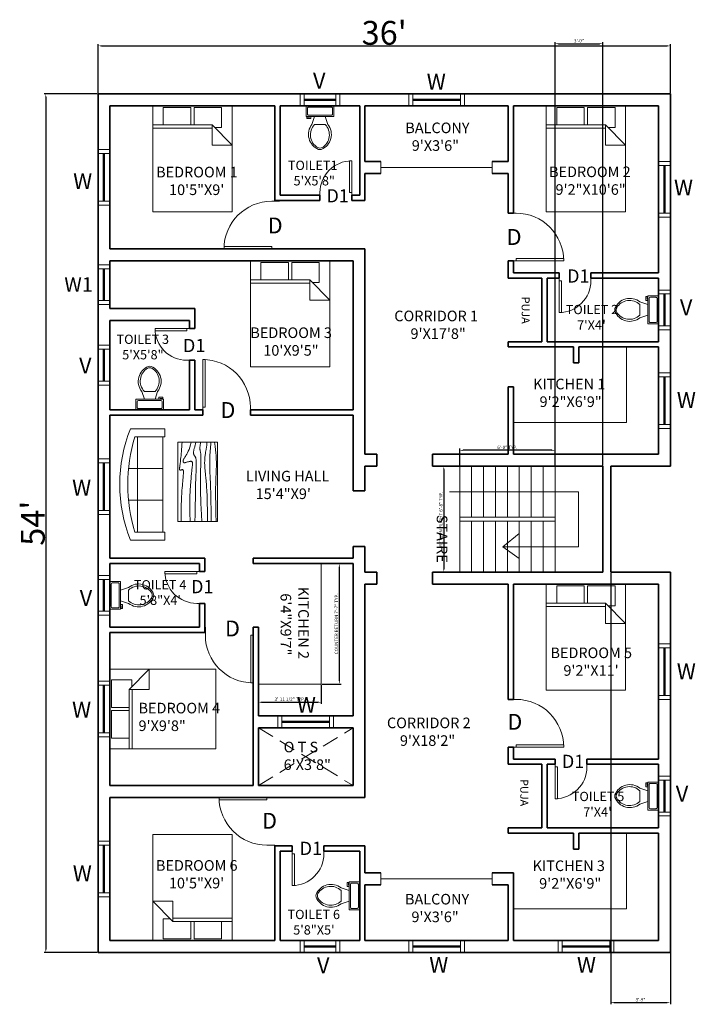
# Model space of a CAD drawing. Units: inches. Extents: x 2391 to 16591, y 7259 to 10239.
# Tile 26 of 27: x 14913 to 15423, y 9413 to 10156. Entities that reach past the tile are written whole.
import ezdxf

# ---------------------------------------------------------------- set-up
doc = ezdxf.new("R2010")
doc.units = ezdxf.units.IN
doc.linetypes.add('DASHED', pattern=[19.05, 12.7, -6.35])
for name, color, linetype, lineweight in [('A-ANNO-DIMS', 4, 'Continuous', 18), ('A-ANNO-IDEN', 2, 'Continuous', 18), ('A-ANNO-SYMB', 3, 'Continuous', 18), ('A-AREA-IDEN', 7, 'Continuous', 18), ('A-DOOR', 3, 'Continuous', 18), ('A-FLOR-CASE', 6, 'Continuous', 18), ('A-FLOR-FIXT', 9, 'Continuous', 18), ('A-FLOR-HRAL', 8, 'Continuous', 18), ('A-FLOR-OPEN', 4, 'DASHED', 13), ('A-FLOR-STRS', 7, 'Continuous', 18), ('A-FURN', 8, 'Continuous', 18), ('A-GLAZ', 4, 'Continuous', 18), ('A-WALL', 7, 'Continuous', 35)]:
    doc.layers.add(name, color=color, linetype=linetype, lineweight=lineweight)
doc.styles.get("Standard").update_dxf_attribs({"font": 'arial.ttf'})
doc.dimstyles.new('ISO-25', dxfattribs={"dimtxt": 2.5, "dimasz": 2.5, "dimexe": 1.25, "dimexo": 0.625, "dimtad": 1, "dimdec": 0, "dimlunit": 3, "dimtxsty": 'Standard', "dimcen": 2.5, "dimadec": 0, "dimazin": 0, "dimtfac": 1, "dimtdec": 0, "dimtmove": 0, "dimatfit": 3, "dimfxl": 1, "dimarcsym": 0})

# ---------------------------------------------------------------- blocks, each defined once
blk = doc.blocks.new('Bed - Queen')
for p, q in [((0, -80.00003), (0, 0)), ((0, 0), (59.99999, 0)), ((59.99999, 0), (59.99999, -80.00003)), ((7.99999, -1.2), (28.79998, -1.2)), ((7.99999, -14.4), (7.99999, -1.2)), ((28.79998, -1.2), (28.79998, -14.4)), ((31.19999, -1.2), (51.99999, -1.2)), ((31.19999, -14.4), (31.19999, -1.2)), ((51.99999, -1.2), (51.99999, -16.4)), ((0, -14.4), (44.8, -14.4)), ((59.99999, -29.6), (44.8, -14.4)), ((44.8, -14.4), (44.8, -29.6)), ((44.8, -16.8), (0, -16.8)), ((51.99999, -16.4), (46.79936, -16.4)), ((44.8, -29.6), (59.99999, -29.6)), ((59.99999, -80.00003), (0, -80.00003))]:
    blk.add_line(p, q)
blk = doc.blocks.new('Toilet - top')
for p, q in [((9.5, -6), (9.5, -2)), ((-10, -8.5), (-8, -8.5)), ((-10, -9.5), (-10, -8.5)), ((-7, -9.5), (-10, -9.5)), ((-8, -8.5), (-8, -8)), ((-7, -8), (-7, -9.5)), ((-4, -8), (-6, -14)), ((4, -14), (-4, -14)), ((4, -8), (6, -14))]:
    blk.add_line(p, q)
blk.add_lwpolyline([(10.5, -8), (10.5, 0), (-10.5, 0), (-10.5, -8)], close=True)
for points in [[(-9.5, -2), (-9.5, -6)], [(8.5, -1), (-8.5, -1)], [(-8.5, -7), (8.5, -7)]]:
    blk.add_lwpolyline(points)
for centre, radius, start, end in [((-8.62, -1.88), 0.884, 81.8699, 188.1301), ((-8.62, -6.12), 0.884, 171.8699, 278.1301), ((8.62, -1.88), 0.884, 351.8699, 98.1301), ((8.62, -6.12), 0.884, 261.8699, 8.1301), ((3.52, -21.58), 12.17, 141.46911, 247.97143), ((4.2, -21.82), 11.33, 136.36773, 238.94682), ((-3.52, -21.58), 12.17, 292.02843, 38.53071), ((-4.2, -21.82), 11.33, 301.05301, 43.63209), ((0, -27.88), 4, 245.73182, 294.26817), ((0, -29), 4, 254.86053, 285.13947)]:
    blk.add_arc(centre, radius, start, end)
blk = doc.blocks.new('Sofa - Roundback 7 ft.')
for p, q in [((-12.00002, -32.4421), (-12.00003, -6.5971)), ((11.99997, -32.4421), (11.99998, -6.5971)), ((-36.000027, -34), (-36.000027, -11.4696)), ((-35.999844, -13.3819), (35.9998, -13.3819)), ((35.99998, -34), (35.99998, -11.4696)), ((-36.000027, -32.4421), (35.99998, -32.4421))]:
    blk.add_line(p, q)
for points in [[(-36.000027, -34), (-42.000027, -34), (-42.000027, -8)], [(41.99998, -8), (41.99998, -34), (35.99998, -34)]]:
    blk.add_lwpolyline(points)
for centre, radius, start, end in [((0, -114.25), 114.25, 68.43141, 111.5686), ((-0.00001, -127.1968), 121.1968, 72.72033, 107.2797)]:
    blk.add_arc(centre, radius, start, end)
blk = doc.blocks.new('Table - Rectangular Woodgrain 60 x 30 in.')
for p, q in [((0, 0), (0, -30)), ((60, 0), (0, 0)), ((60, -30), (60, 0)), ((0, -30), (60, -30))]:
    blk.add_line(p, q)
for points in [[(0, -2.4), (4.8155, -2.418), (9.0302, -2.4688), (12.709, -2.5477), (15.9167, -2.65), (18.7181, -2.7711), (21.1781, -2.9063), (23.3616, -3.0508), (25.3333, -3.2), (27.1477, -3.3495), (28.8172, -3.4958), (30.3437, -3.636), (31.7291, -3.7667), (32.9756, -3.8849), (34.0849, -3.9875), (35.059, -4.0714), (35.9, -4.1334), (36.6114, -4.1711), (37.2041, -4.1854), (37.6906, -4.1779), (38.0833, -4.15), (38.3948, -4.1034), (38.6375, -4.0396), (38.8239, -3.9602), (38.9666, -3.8667), (39.0764, -3.7608), (39.1573, -3.6448), (39.2116, -3.521), (39.2416, -3.3917), (39.2498, -3.2593), (39.2385, -3.1261), (39.21, -2.9944), (39.1666, -2.8667), (39.111, -2.7447), (39.0468, -2.6281), (38.978, -2.5163), (38.9083, -2.4083), (38.8418, -2.3035), (38.7823, -2.201), (38.7337, -2.1001), (38.7, -2), (38.6844, -1.9003), (38.6875, -1.8021), (38.7094, -1.707), (38.75, -1.6167), (38.8094, -1.5326), (38.8875, -1.4563), (38.9844, -1.3893), (39.1, -1.3333), (39.2351, -1.2896), (39.3937, -1.2583), (39.5804, -1.2396), (39.8, -1.2333), (40.057, -1.2396), (40.3562, -1.2583), (40.7023, -1.2896), (41.1, -1.3333), (41.5547, -1.3895), (42.0755, -1.4573), (42.6721, -1.5361), (43.3542, -1.625), (44.1316, -1.7233), (45.014, -1.8302), (46.0114, -1.9449), (47.1333, -2.0667), (48.3862, -2.1947), (49.7625, -2.3281), (51.2513, -2.4663), (52.8416, -2.6083), (54.5226, -2.7535), (56.2833, -2.9011), (58.1127, -3.0501), (60, -3.2)], [(0, -9.2), (6.5759, -9.0858), (11.9385, -9.0365), (16.2527, -9.0418), (19.6833, -9.0917), (22.3952, -9.1759), (24.5531, -9.2844), (26.322, -9.4069), (27.8666, -9.5333), (29.3241, -9.6553), (30.7203, -9.7719), (32.0532, -9.8837), (33.3208, -9.9917), (34.5213, -10.0965), (35.6526, -10.199), (36.7128, -10.2999), (37.7, -10.4), (38.6129, -10.4996), (39.4531, -10.5969), (40.223, -10.6895), (40.925, -10.775), (41.5613, -10.8512), (42.1344, -10.9156), (42.6465, -10.966), (43.1, -11), (43.4976, -11.0158), (43.8437, -11.0136), (44.143, -10.9942), (44.4, -10.9583), (44.6195, -10.9069), (44.8062, -10.8406), (44.9648, -10.7603), (45.1, -10.6667), (45.2155, -10.5598), (45.3114, -10.4365), (45.3871, -10.2929), (45.4416, -10.125), (45.4743, -9.929), (45.4844, -9.7011), (45.4709, -9.4371), (45.4333, -9.1333), (45.3716, -8.7883), (45.2896, -8.4104), (45.1919, -8.0107), (45.0833, -7.6), (44.9685, -7.1893), (44.8521, -6.7896), (44.7388, -6.4117), (44.6333, -6.0667), (44.54, -5.7628), (44.4614, -5.4979), (44.4001, -5.2675), (44.3583, -5.0667), (44.3384, -4.8909), (44.3427, -4.7354), (44.3736, -4.5956), (44.4333, -4.4667), (44.5236, -4.3453), (44.6427, -4.2333), (44.7884, -4.1339), (44.9583, -4.05), (45.1501, -3.9849), (45.3614, -3.9417), (45.59, -3.9234), (45.8333, -3.9333), (46.0915, -3.9749), (46.3734, -4.0531), (46.6906, -4.1736), (47.0542, -4.3417), (47.4756, -4.5629), (47.9661, -4.8427), (48.5372, -5.1866), (49.2, -5.6), (49.9676, -6.0844), (50.8594, -6.625), (51.8965, -7.2031), (53.1, -7.8), (54.491, -8.3969), (56.0906, -8.975), (57.9199, -9.5156), (60, -10)], [(0, -12.8), (5.1847, -12.9322), (9.6213, -13.0323), (13.3963, -13.1059), (16.5958, -13.1583), (19.3063, -13.1952), (21.614, -13.2219), (23.6054, -13.2439), (25.3666, -13.2667), (26.9728, -13.2947), (28.4531, -13.3281), (29.8256, -13.3663), (31.1083, -13.4083), (32.3191, -13.4535), (33.476, -13.501), (34.597, -13.5501), (35.7, -13.6), (36.7984, -13.6497), (37.8875, -13.6979), (38.9578, -13.743), (40, -13.7833), (41.0047, -13.8174), (41.9625, -13.8438), (42.864, -13.8607), (43.7, -13.8667), (44.4631, -13.8604), (45.1552, -13.8417), (45.7801, -13.8104), (46.3416, -13.7667), (46.8439, -13.7104), (47.2906, -13.6417), (47.6858, -13.5604), (48.0333, -13.4667), (48.3375, -13.3608), (48.6042, -13.2448), (48.8396, -13.121), (49.05, -12.9917), (49.2417, -12.8593), (49.4208, -12.7261), (49.5937, -12.5944), (49.7667, -12.4667), (49.9452, -12.3451), (50.1323, -12.2313), (50.3303, -12.1268), (50.5416, -12.0333), (50.7686, -11.9524), (51.0135, -11.8854), (51.2788, -11.8341), (51.5666, -11.8), (51.8785, -11.7843), (52.2116, -11.7865), (52.562, -11.8059), (52.926, -11.8417), (53.2998, -11.8931), (53.6795, -11.9594), (54.0614, -12.0397), (54.4416, -12.1333), (54.8223, -12.2401), (55.2293, -12.3625), (55.6942, -12.5037), (56.2489, -12.6667), (56.9251, -12.8547), (57.7545, -13.0708), (58.7689, -13.3182), (60, -13.6)], [(0, -18), (5.124, -17.7273), (9.6609, -17.5057), (13.6705, -17.3303), (17.2125, -17.1958), (20.3467, -17.0973), (23.1328, -17.0297), (25.6307, -16.9878), (27.9, -16.9667), (29.9928, -16.9617), (31.9302, -16.9703), (33.7254, -16.9907), (35.3917, -17.0208), (36.9423, -17.0588), (38.3906, -17.1026), (39.7499, -17.1503), (41.0333, -17.2), (42.2519, -17.2496), (43.4073, -17.2969), (44.4986, -17.3395), (45.525, -17.375), (46.4858, -17.4012), (47.3802, -17.4156), (48.2074, -17.416), (48.9667, -17.4), (49.6583, -17.3662), (50.2872, -17.3167), (50.8595, -17.2547), (51.3812, -17.1833), (51.8584, -17.1057), (52.2971, -17.025), (52.7034, -16.9443), (53.0833, -16.8667), (53.443, -16.7951), (53.789, -16.7313), (54.128, -16.6768), (54.4666, -16.6334), (54.8115, -16.6024), (55.1693, -16.5854), (55.5465, -16.5841), (55.95, -16.6), (56.3828, -16.6337), (56.8346, -16.6823), (57.2915, -16.7418), (57.7396, -16.8084), (58.165, -16.878), (58.5539, -16.9469), (58.8924, -17.0111), (59.1666, -17.0667), (59.3679, -17.1107), (59.5078, -17.1438), (59.6032, -17.1675), (59.6708, -17.1833), (59.7275, -17.193), (59.7901, -17.1979), (59.8753, -17.1998), (60, -17.2)], [(0, -22.4), (8.0098, -22.2501), (14.4094, -22.1011), (19.4168, -21.9535), (23.25, -21.8083), (26.1269, -21.6663), (28.2656, -21.5281), (29.884, -21.3947), (31.2, -21.2667), (32.3967, -21.1448), (33.5172, -21.0292), (34.5697, -20.9198), (35.5625, -20.8167), (36.5037, -20.7198), (37.4015, -20.6292), (38.2642, -20.5448), (39.1, -20.4667), (39.9164, -20.3951), (40.7187, -20.3313), (41.5117, -20.2768), (42.3, -20.2333), (43.0883, -20.2024), (43.8812, -20.1854), (44.6836, -20.1841), (45.5, -20.2), (46.3328, -20.234), (47.1747, -20.2844), (48.0163, -20.3488), (48.8479, -20.425), (49.66, -20.5106), (50.4429, -20.6031), (51.1872, -20.7004), (51.8833, -20.8), (52.5246, -20.8999), (53.1166, -20.9995), (53.6681, -21.0983), (54.1875, -21.1958), (54.6834, -21.2919), (55.1646, -21.3859), (55.6394, -21.4777), (56.1167, -21.5667), (56.6028, -21.6515), (57.0961, -21.7266), (57.5929, -21.7852), (58.0896, -21.8208), (58.5823, -21.8268), (59.0674, -21.7964), (59.5412, -21.723), (60, -21.6)], [(0, -25.2), (8.6355, -25.0504), (15.7026, -24.9031), (21.4049, -24.7606), (25.9458, -24.625), (29.529, -24.4988), (32.3578, -24.3844), (34.6359, -24.284), (36.5667, -24.2), (38.3213, -24.1341), (39.9417, -24.0854), (41.437, -24.0523), (42.8167, -24.0333), (44.0901, -24.0268), (45.2667, -24.0313), (46.3557, -24.0451), (47.3667, -24.0667), (48.309, -24.0947), (49.1928, -24.1287), (50.0284, -24.168), (50.826, -24.2125), (51.5959, -24.2617), (52.3483, -24.3151), (53.0935, -24.3725), (53.8417, -24.4334), (54.6009, -24.497), (55.3699, -24.561), (56.1454, -24.6226), (56.9239, -24.6792), (57.7021, -24.7279), (58.4764, -24.7662), (59.2435, -24.7911), (60, -24.8)], [(0, -28.8), (5.6867, -28.6681), (10.45, -28.5698), (14.407, -28.5012), (17.675, -28.4584), (20.3711, -28.4374), (22.6125, -28.4344), (24.5164, -28.4455), (26.2, -28.4667), (27.762, -28.4947), (29.2276, -28.5281), (30.6033, -28.5663), (31.8958, -28.6084), (33.1118, -28.6535), (34.2578, -28.7011), (35.3405, -28.7501), (36.3666, -28.8), (37.3443, -28.8497), (38.288, -28.8974), (39.2137, -28.9412), (40.1375, -28.9792), (41.0753, -29.0093), (42.0432, -29.0297), (43.0572, -29.0384), (44.1333, -29.0333), (45.2936, -29.0114), (46.5843, -28.9641), (48.0579, -28.8816), (49.7666, -28.7542), (51.7629, -28.5721), (54.0989, -28.3255), (56.8272, -28.0048), (60, -27.6)]]:
    blk.add_lwpolyline(points)
blk = doc.blocks.new('*U7')
for p, q in [((0, 0), (0, -6)), ((36, 0), (36, -6))]:
    blk.add_line(p, q)
blk.add_lwpolyline([(0, 0), (0, 36), (1.75, 36), (1.75, 0)], close=True)
blk.add_arc((0, 0), 36, 0, 90)
blk = doc.blocks.new('*U6')
for p, q in [((-36, 0), (-36, 6)), ((0, 0), (0, 6))]:
    blk.add_line(p, q)
blk.add_lwpolyline([(0, 0), (0, -36), (-1.75, -36), (-1.75, 0)], close=True)
blk.add_arc((0, 0), 36, 180, 270)
blk = doc.blocks.new('*U8')
for p, q in [((-24, 0), (-24, -6)), ((0, 0), (0, -6))]:
    blk.add_line(p, q)
blk.add_lwpolyline([(0, 0), (0, 24), (-1.75, 24), (-1.75, 0)], close=True)
blk.add_arc((0, 0), 24, 90, 180)
blk = doc.blocks.new('*U9')
for p, q in [((0, 0), (0, 6)), ((24, 0), (24, 6))]:
    blk.add_line(p, q)
blk.add_lwpolyline([(0, 0), (0, -24), (1.75, -24), (1.75, 0)], close=True)
blk.add_arc((0, 0), 24, 270, 0)
blk = doc.blocks.new('*U10')
for p, q in [((0, 0), (0, -6)), ((-36, 0), (-36, -6))]:
    blk.add_line(p, q)
blk.add_lwpolyline([(0, 0), (0, 36), (-1.75, 36), (-1.75, 0)], close=True)
blk.add_arc((0, 0), 36, 90, 180)
blk = doc.blocks.new('*U11')
for p, q in [((-36, 0), (-36, 6)), ((0, 0), (0, 6))]:
    blk.add_line(p, q)
blk.add_lwpolyline([(0, 0), (0, -36), (-1.75, -36), (-1.75, 0)], close=True)
blk.add_arc((0, 0), 36, 180, 270)
blk = doc.blocks.new('*U12')
for p, q in [((0, 0), (0, -6)), ((-36, 0), (-36, -6))]:
    blk.add_line(p, q)
blk.add_lwpolyline([(0, 0), (0, 36), (-1.75, 36), (-1.75, 0)], close=True)
blk.add_arc((0, 0), 36, 90, 180)
blk = doc.blocks.new('*U13')
for p, q in [((0, 0), (0, 6)), ((36, 0), (36, 6))]:
    blk.add_line(p, q)
blk.add_lwpolyline([(0, 0), (0, -36), (1.75, -36), (1.75, 0)], close=True)
blk.add_arc((0, 0), 36, 270, 0)
blk = doc.blocks.new('*D21')
at = {"layer": 'A-ANNO-DIMS', "color": 0, "lineweight": -2, "transparency": 16777216}
for p, q in [((14971.9, 10100.91), (14971.9, 10137.81)), ((15403.9, 10100.91), (15403.9, 10137.81)), ((14974.4, 10136.56), (15401.4, 10136.56))]:
    blk.add_line(p, q, dxfattribs=at)
at = {"layer": 'A-ANNO-DIMS', "color": 0, "transparency": 16777216}
for points in [[(14974.4, 10136.98), (14974.4, 10136.15), (14971.9, 10136.56)], [(15401.4, 10136.98), (15401.4, 10136.15), (15403.9, 10136.56)]]:
    blk.add_solid(points, dxfattribs=at)
at = {"layer": 'Defpoints', "color": 0, "transparency": 16777216}
for p in [(15403.9, 10136.56), (14971.9, 10100.28), (15403.9, 10100.28)]:
    blk.add_point(p, dxfattribs=at)
at = {"layer": 'A-ANNO-DIMS', "color": 0, "transparency": 16777216, "insert": (15187.9, 10146.39), "char_height": 2.5, "attachment_point": 5}
blk.add_mtext("{\\H7.2x;36'}", dxfattribs=at)
blk = doc.blocks.new('*D22')
at = {"layer": 'A-ANNO-DIMS', "color": 0, "lineweight": -2, "transparency": 16777216}
for p, q in [((14971.27, 10100.28), (14931.23, 10100.28)), ((14932.48, 10097.78), (14932.48, 9454.78)), ((14971.27, 9452.28), (14931.23, 9452.28))]:
    blk.add_line(p, q, dxfattribs=at)
at = {"layer": 'A-ANNO-DIMS', "color": 0, "transparency": 16777216}
for points in [[(14932.06, 10097.78), (14932.9, 10097.78), (14932.48, 10100.28)], [(14932.06, 9454.78), (14932.9, 9454.78), (14932.48, 9452.28)]]:
    blk.add_solid(points, dxfattribs=at)
at = {"layer": 'Defpoints', "color": 0, "transparency": 16777216}
for p in [(14971.9, 10100.28), (14932.48, 9452.28), (14971.9, 9452.28)]:
    blk.add_point(p, dxfattribs=at)
at = {"layer": 'A-ANNO-DIMS', "color": 0, "transparency": 16777216, "insert": (14922.7, 9776.28), "char_height": 2.5, "attachment_point": 5, "rotation": 90}
blk.add_mtext("{\\H7.2x;54'}", dxfattribs=at)
blk = doc.blocks.new('WINDOW-36-PLAN')
for p, q in [((9, 42), (0, 42)), ((9, 39), (0, 39)), ((4, 39), (4, 3)), ((4.5, 39), (4.5, 3)), ((5, 39), (5, 3)), ((9, 3), (0, 3)), ((9, 0), (0, 0))]:
    blk.add_line(p, q)
blk = doc.blocks.new('VENT-24-PLAN')
for p, q in [((9, 30), (0, 30)), ((9, 27), (0, 27)), ((4, 27), (4, 3)), ((4.5, 27), (4.5, 3)), ((5, 27), (5, 3)), ((9, 3), (0, 3)), ((9, 0), (0, 0))]:
    blk.add_line(p, q)
blk = doc.blocks.new('WINDOW-24-PLAN')
for p, q in [((9, 30), (0, 30)), ((9, 27), (0, 27)), ((4, 27), (4, 3)), ((4.5, 27), (4.5, 3)), ((5, 27), (5, 3)), ((9, 3), (0, 3)), ((9, 0), (0, 0))]:
    blk.add_line(p, q)
blk = doc.blocks.new('STAIR-RETURN-FLIGHT')
for p, q in [((0, 80), (0, 0)), ((9, 80), (9, 41.5)), ((18, 80), (18, 41.5)), ((27, 80), (27, 41.5)), ((36, 80), (36, 41.5)), ((45, 80), (45, 41.5)), ((54, 80), (54, 41.5)), ((63, 80), (63, 41.5)), ((72, 80), (72, 0)), ((72, 41.5), (0, 41.5)), ((72, 38.5), (0, 38.5)), ((9, 38.5), (9, 0)), ((18, 38.5), (18, 0)), ((27, 38.5), (27, 0)), ((36, 38.5), (36, 0)), ((45, 38.5), (45, 0)), ((54, 38.5), (54, 0)), ((63, 38.5), (63, 0))]:
    blk.add_line(p, q)
blk = doc.blocks.new('STAIR-DIRECTION-ARROW')
for p, q in [((0, 50.31), (97.37, 50.31)), ((97.37, 50.31), (97.37, 8.81)), ((40.34, 8.81), (52.74, 18.89)), ((97.37, 8.81), (40.34, 8.81)), ((40.34, 8.81), (52.74, 0))]:
    blk.add_line(p, q)
blk = doc.blocks.new('COUNTER-L-RETURN')
for q in [(47.5, 91), (0, 0)]:
    blk.add_line((47.5, 0), q)
blk = doc.blocks.new('COUNTER-L-KITCHEN')
for p, q in [((85.5, 57), (85.5, 0)), ((85.5, 0), (0, 0))]:
    blk.add_line(p, q)
blk = doc.blocks.new('*D57')
at = {"layer": 'A-ANNO-DIMS', "color": 0, "lineweight": -2, "transparency": 16777216}
for p, q in [((15141.02, 9745.78), (15155.3, 9745.78)), ((15154.05, 9657.28), (15154.05, 9743.28)), ((15141.02, 9654.78), (15155.3, 9654.78))]:
    blk.add_line(p, q, dxfattribs=at)
at = {"layer": 'A-ANNO-DIMS', "color": 0, "transparency": 16777216}
for points in [[(15153.63, 9743.28), (15154.46, 9743.28), (15154.05, 9745.78)], [(15153.63, 9657.28), (15154.46, 9657.28), (15154.05, 9654.78)]]:
    blk.add_solid(points, dxfattribs=at)
at = {"layer": 'Defpoints', "color": 0, "transparency": 16777216}
for p in [(15140.4, 9745.78), (15154.05, 9745.78), (15140.4, 9654.78)]:
    blk.add_point(p, dxfattribs=at)
at = {"layer": 'A-ANNO-DIMS', "color": 0, "transparency": 16777216, "insert": (15152.13, 9700.28), "char_height": 2.5, "attachment_point": 5, "rotation": 90}
blk.add_mtext('COUNTER RETURN 7\'-7" TYP.', dxfattribs=at)
blk = doc.blocks.new('*D58')
at = {"layer": 'A-ANNO-DIMS', "color": 0, "lineweight": -2, "transparency": 16777216}
for p, q in [((15092.9, 9654.16), (15092.9, 9639.88)), ((15140.4, 9654.16), (15140.4, 9639.88)), ((15095.4, 9641.13), (15137.9, 9641.13))]:
    blk.add_line(p, q, dxfattribs=at)
at = {"layer": 'A-ANNO-DIMS', "color": 0, "transparency": 16777216}
for points in [[(15095.4, 9641.55), (15095.4, 9640.71), (15092.9, 9641.13)], [(15137.9, 9641.55), (15137.9, 9640.71), (15140.4, 9641.13)]]:
    blk.add_solid(points, dxfattribs=at)
at = {"layer": 'Defpoints', "color": 0, "transparency": 16777216}
for p in [(15092.9, 9654.78), (15140.4, 9654.78), (15140.4, 9641.13)]:
    blk.add_point(p, dxfattribs=at)
at = {"layer": 'A-ANNO-DIMS', "color": 0, "transparency": 16777216, "insert": (15116.65, 9643.05), "char_height": 2.5, "attachment_point": 5}
blk.add_mtext('3\'-11 1/2" TYP.', dxfattribs=at)
blk = doc.blocks.new('*D59')
at = {"layer": 'A-ANNO-DIMS', "color": 0, "lineweight": -2, "transparency": 16777216}
for p, q in [((15244.27, 9819.28), (15231.65, 9819.28)), ((15232.9, 9816.78), (15232.9, 9741.78)), ((15244.27, 9739.28), (15231.65, 9739.28))]:
    blk.add_line(p, q, dxfattribs=at)
at = {"layer": 'A-ANNO-DIMS', "color": 0, "transparency": 16777216}
for points in [[(15232.48, 9816.78), (15233.31, 9816.78), (15232.9, 9819.28)], [(15232.48, 9741.78), (15233.31, 9741.78), (15232.9, 9739.28)]]:
    blk.add_solid(points, dxfattribs=at)
at = {"layer": 'Defpoints', "color": 0, "transparency": 16777216}
for p in [(15244.9, 9819.28), (15232.9, 9739.28), (15244.9, 9739.28)]:
    blk.add_point(p, dxfattribs=at)
at = {"layer": 'A-ANNO-DIMS', "color": 0, "transparency": 16777216, "insert": (15230.98, 9779.28), "char_height": 2.5, "attachment_point": 5, "rotation": 90}
blk.add_mtext('RETURN FLIGHT 6\'-8" TYP.', dxfattribs=at)
blk = doc.blocks.new('*D60')
at = {"layer": 'A-ANNO-DIMS', "color": 0, "lineweight": -2, "transparency": 16777216}
for p, q in [((15244.9, 9819.91), (15244.9, 9832.53)), ((15316.9, 9819.91), (15316.9, 9832.53)), ((15314.4, 9831.28), (15247.4, 9831.28))]:
    blk.add_line(p, q, dxfattribs=at)
at = {"layer": 'A-ANNO-DIMS', "color": 0, "transparency": 16777216}
for points in [[(15247.4, 9831.7), (15247.4, 9830.86), (15244.9, 9831.28)], [(15314.4, 9831.7), (15314.4, 9830.86), (15316.9, 9831.28)]]:
    blk.add_solid(points, dxfattribs=at)
at = {"layer": 'Defpoints', "color": 0, "transparency": 16777216}
for p in [(15244.9, 9831.28), (15244.9, 9819.28), (15316.9, 9819.28)]:
    blk.add_point(p, dxfattribs=at)
at = {"layer": 'A-ANNO-DIMS', "color": 0, "transparency": 16777216, "insert": (15280.9, 9833.18), "char_height": 2.5, "attachment_point": 5}
blk.add_mtext('6\'-0" TYP.', dxfattribs=at)
blk = doc.blocks.new('*D72')
at = {"layer": 'A-ANNO-DIMS', "color": 0, "lineweight": -2, "transparency": 16777216}
for p, q in [((15316.9, 9819.91), (15316.9, 10139.43)), ((15319.4, 10138.18), (15350.4, 10138.18)), ((15352.9, 9819.91), (15352.9, 10139.43))]:
    blk.add_line(p, q, dxfattribs=at)
at = {"layer": 'A-ANNO-DIMS', "color": 0, "transparency": 16777216}
for points in [[(15319.4, 10138.6), (15319.4, 10137.76), (15316.9, 10138.18)], [(15350.4, 10138.6), (15350.4, 10137.76), (15352.9, 10138.18)]]:
    blk.add_solid(points, dxfattribs=at)
at = {"layer": 'Defpoints', "color": 0, "transparency": 16777216}
for p in [(15352.9, 10138.18), (15316.9, 9819.28), (15352.9, 9819.28)]:
    blk.add_point(p, dxfattribs=at)
at = {"layer": 'A-ANNO-DIMS', "color": 0, "transparency": 16777216, "insert": (15334.9, 10140.08), "char_height": 2.5, "attachment_point": 5}
blk.add_mtext('3\'-0"', dxfattribs=at)
blk = doc.blocks.new('*D73')
at = {"layer": 'A-ANNO-DIMS', "color": 0, "lineweight": -2, "transparency": 16777216}
for p, q in [((15358.9, 9738.66), (15358.9, 9413.13)), ((15403.9, 9738.66), (15403.9, 9413.13)), ((15361.4, 9414.38), (15401.4, 9414.38))]:
    blk.add_line(p, q, dxfattribs=at)
at = {"layer": 'A-ANNO-DIMS', "color": 0, "transparency": 16777216}
for points in [[(15361.4, 9414.8), (15361.4, 9413.96), (15358.9, 9414.38)], [(15401.4, 9414.8), (15401.4, 9413.96), (15403.9, 9414.38)]]:
    blk.add_solid(points, dxfattribs=at)
at = {"layer": 'Defpoints', "color": 0, "transparency": 16777216}
for p in [(15358.9, 9739.28), (15403.9, 9739.28), (15403.9, 9414.38)]:
    blk.add_point(p, dxfattribs=at)
at = {"layer": 'A-ANNO-DIMS', "color": 0, "transparency": 16777216, "insert": (15381.4, 9416.28), "char_height": 2.5, "attachment_point": 5}
blk.add_mtext('3\'-9"', dxfattribs=at)

msp = doc.modelspace()

# ---------------------------------------------------------------- linework, layer by layer
at = {"layer": 'A-DOOR'}
msp.add_line((15105.25, 9569.28), (15105.25, 9569.28), dxfattribs=at)
at = {"layer": 'A-FLOR-HRAL'}
for p, q in [((15185.4, 10040.28), (15185.4, 10049.28)), ((15269.4, 10040.28), (15269.4, 10049.28)), ((15185.4, 10044.78), (15269.4, 10044.78)), ((15185.4, 9503.28), (15185.4, 9512.28)), ((15185.4, 9507.78), (15269.4, 9507.78)), ((15269.4, 9503.28), (15269.4, 9512.28))]:
    msp.add_line(p, q, dxfattribs=at)
at = {"layer": 'A-FLOR-OPEN'}
for p, q in [((15092.9, 9578.28), (15164.4, 9621.78)), ((15092.9, 9621.78), (15164.4, 9578.28))]:
    msp.add_line(p, q, dxfattribs=at)
at = {"layer": 'A-WALL'}
for p, q in [((14971.9, 10100.28), (15403.9, 10100.28)), ((14971.9, 9452.28), (14971.9, 10100.28)), ((15403.9, 10100.28), (15403.9, 9819.28)), ((14980.9, 10091.28), (15105.4, 10091.28)), ((14980.9, 9983.28), (14980.9, 10091.28)), ((15105.4, 10019.78), (15105.4, 10091.28)), ((15109.4, 10091.28), (15169.4, 10091.28)), ((15109.4, 10023.78), (15109.4, 10091.28)), ((15169.4, 10023.78), (15169.4, 10091.28)), ((15173.4, 10091.28), (15281.4, 10091.28)), ((15173.4, 10049.28), (15173.4, 10091.28)), ((15281.4, 10049.28), (15281.4, 10091.28)), ((15285.4, 10091.28), (15394.9, 10091.28)), ((15285.4, 10010.28), (15285.4, 10091.28)), ((15394.9, 10091.28), (15394.9, 9965.28)), ((15173.4, 10049.28), (15185.4, 10049.28)), ((15269.4, 10049.28), (15281.4, 10049.28)), ((15173.4, 10040.28), (15185.4, 10040.28)), ((15173.4, 10019.78), (15173.4, 10040.28)), ((15269.4, 10040.28), (15281.4, 10040.28)), ((15281.4, 10010.28), (15281.4, 10040.28)), ((15105.4, 10019.78), (15139.4, 10019.78)), ((15109.4, 10023.78), (15139.4, 10023.78)), ((15139.4, 10019.78), (15139.4, 10023.78)), ((15163.4, 10023.78), (15169.4, 10023.78)), ((15163.4, 10019.78), (15163.4, 10023.78)), ((15163.4, 10019.78), (15173.4, 10019.78)), ((15281.4, 10010.28), (15285.4, 10010.28)), ((14980.9, 9983.28), (15173.4, 9983.28)), ((15173.4, 9828.28), (15173.4, 9983.28)), ((14980.9, 9974.28), (15164.4, 9974.28)), ((14980.9, 9938.28), (14980.9, 9974.28)), ((15164.4, 9861.78), (15164.4, 9974.28)), ((15281.4, 9974.28), (15285.4, 9974.28)), ((15281.4, 9961.28), (15281.4, 9974.28)), ((15285.4, 9965.28), (15285.4, 9974.28)), ((15281.4, 9961.28), (15306.9, 9961.28)), ((15285.4, 9965.28), (15319.9, 9965.28)), ((15306.9, 9961.28), (15306.9, 9913.28)), ((15310.9, 9961.28), (15319.9, 9961.28)), ((15310.9, 9961.28), (15310.9, 9913.28)), ((15319.9, 9965.28), (15319.9, 9961.28)), ((15343.9, 9965.28), (15394.9, 9965.28)), ((15343.9, 9965.28), (15343.9, 9961.28)), ((15343.9, 9961.28), (15394.9, 9961.28)), ((15394.9, 9961.28), (15394.9, 9913.28)), ((14980.9, 9938.28), (15044.9, 9938.28)), ((15044.9, 9923.28), (15044.9, 9938.28)), ((14980.9, 9929.28), (15040.9, 9929.28)), ((14980.9, 9861.78), (14980.9, 9929.28)), ((15040.9, 9923.28), (15040.9, 9929.28)), ((15040.9, 9923.28), (15044.9, 9923.28)), ((15281.4, 9913.28), (15306.9, 9913.28)), ((15281.4, 9909.28), (15281.4, 9913.28)), ((15281.4, 9909.28), (15330.9, 9909.28)), ((15310.9, 9913.28), (15394.9, 9913.28)), ((15330.9, 9909.28), (15330.9, 9897.28)), ((15334.9, 9909.28), (15394.9, 9909.28)), ((15334.9, 9909.28), (15334.9, 9897.28)), ((15394.9, 9909.28), (15394.9, 9828.28)), ((15040.9, 9899.28), (15044.9, 9899.28)), ((15040.9, 9861.78), (15040.9, 9899.28)), ((15044.9, 9861.78), (15044.9, 9899.28)), ((15330.9, 9897.28), (15334.9, 9897.28)), ((15281.4, 9879.28), (15285.4, 9879.28)), ((15281.4, 9828.28), (15281.4, 9879.28)), ((15285.4, 9828.28), (15285.4, 9879.28)), ((14980.9, 9861.78), (15040.9, 9861.78)), ((14980.9, 9857.78), (15050.9, 9857.78)), ((14980.9, 9749.78), (14980.9, 9857.78)), ((15044.9, 9861.78), (15050.9, 9861.78)), ((15050.9, 9857.78), (15050.9, 9861.78)), ((15086.9, 9861.78), (15164.4, 9861.78)), ((15086.9, 9857.78), (15086.9, 9861.78)), ((15086.9, 9857.78), (15164.4, 9857.78)), ((15164.4, 9800.78), (15164.4, 9857.78)), ((15173.4, 9828.28), (15182.4, 9828.28)), ((15182.4, 9819.28), (15182.4, 9828.28)), ((15224.4, 9828.28), (15281.4, 9828.28)), ((15224.4, 9819.28), (15224.4, 9828.28)), ((15285.4, 9828.28), (15394.9, 9828.28)), ((15173.4, 9819.28), (15182.4, 9819.28)), ((15173.4, 9800.78), (15173.4, 9819.28)), ((15224.4, 9819.28), (15352.9, 9819.28)), ((15352.9, 9819.28), (15352.9, 9739.28)), ((15358.9, 9819.28), (15403.9, 9819.28)), ((15358.9, 9819.28), (15358.9, 9739.28)), ((15164.4, 9800.78), (15173.4, 9800.78)), ((15164.4, 9758.78), (15173.4, 9758.78)), ((15164.4, 9749.78), (15164.4, 9758.78)), ((15173.4, 9739.28), (15173.4, 9758.78)), ((14980.9, 9749.78), (15052.4, 9749.78)), ((14980.9, 9745.78), (15048.4, 9745.78)), ((14980.9, 9697.78), (14980.9, 9745.78)), ((15048.4, 9739.78), (15048.4, 9745.78)), ((15052.4, 9739.78), (15052.4, 9749.78)), ((15088.9, 9749.78), (15164.4, 9749.78)), ((15088.9, 9745.78), (15088.9, 9749.78)), ((15088.9, 9745.78), (15164.4, 9745.78)), ((15164.4, 9630.78), (15164.4, 9745.78)), ((15048.4, 9739.78), (15052.4, 9739.78)), ((15182.4, 9739.28), (15173.4, 9739.28)), ((15182.4, 9730.28), (15182.4, 9739.28)), ((15352.9, 9739.28), (15224.4, 9739.28)), ((15224.4, 9730.28), (15224.4, 9739.28)), ((15403.9, 9739.28), (15358.9, 9739.28)), ((15403.9, 9739.28), (15403.9, 9452.28)), ((15182.4, 9730.28), (15173.4, 9730.28)), ((15173.4, 9569.28), (15173.4, 9730.28)), ((15281.4, 9730.28), (15224.4, 9730.28)), ((15281.4, 9643.28), (15281.4, 9730.28)), ((15394.9, 9730.28), (15285.4, 9730.28)), ((15285.4, 9643.28), (15285.4, 9730.28)), ((15394.9, 9730.28), (15394.9, 9598.28)), ((15048.4, 9715.78), (15052.4, 9715.78)), ((15048.4, 9697.78), (15048.4, 9715.78)), ((15052.4, 9693.78), (15052.4, 9715.78)), ((14980.9, 9697.78), (15048.4, 9697.78)), ((14980.9, 9693.78), (15052.4, 9693.78)), ((14980.9, 9578.28), (14980.9, 9693.78)), ((15088.9, 9697.78), (15092.9, 9697.78)), ((15088.9, 9578.28), (15088.9, 9697.78)), ((15092.9, 9630.78), (15092.9, 9697.78)), ((15285.4, 9643.28), (15281.4, 9643.28)), ((15164.4, 9630.78), (15092.9, 9630.78)), ((15164.4, 9621.78), (15092.9, 9621.78)), ((15092.9, 9578.28), (15092.9, 9621.78)), ((15164.4, 9578.28), (15164.4, 9621.78)), ((15285.4, 9607.28), (15281.4, 9607.28)), ((15281.4, 9594.28), (15281.4, 9607.28)), ((15285.4, 9598.28), (15285.4, 9607.28)), ((15316.9, 9598.28), (15285.4, 9598.28)), ((15316.9, 9598.28), (15316.9, 9594.28)), ((15340.9, 9598.28), (15340.9, 9594.28)), ((15394.9, 9598.28), (15340.9, 9598.28)), ((15306.9, 9594.28), (15281.4, 9594.28)), ((15306.9, 9594.28), (15306.9, 9546.28)), ((15310.9, 9594.28), (15310.9, 9546.28)), ((15316.9, 9594.28), (15310.9, 9594.28)), ((15394.9, 9594.28), (15340.9, 9594.28)), ((15394.9, 9594.28), (15394.9, 9546.28)), ((15088.9, 9578.28), (14980.9, 9578.28)), ((15164.4, 9578.28), (15092.9, 9578.28)), ((15109.4, 9569.28), (14980.9, 9569.28)), ((14980.9, 9461.28), (14980.9, 9569.28)), ((15173.4, 9569.28), (15109.4, 9569.28)), ((15306.9, 9546.28), (15281.4, 9546.28)), ((15281.4, 9542.28), (15281.4, 9546.28)), ((15394.9, 9546.28), (15310.9, 9546.28)), ((15330.9, 9542.28), (15281.4, 9542.28)), ((15330.9, 9542.28), (15330.9, 9530.28)), ((15334.9, 9542.28), (15334.9, 9530.28)), ((15394.9, 9542.28), (15334.9, 9542.28)), ((15394.9, 9542.28), (15394.9, 9461.28)), ((15118.4, 9532.78), (15105.4, 9532.78)), ((15105.4, 9461.28), (15105.4, 9532.78)), ((15118.4, 9528.78), (15109.4, 9528.78)), ((15109.4, 9461.28), (15109.4, 9528.78)), ((15118.4, 9528.78), (15118.4, 9532.78)), ((15173.4, 9532.78), (15142.4, 9532.78)), ((15142.4, 9528.78), (15142.4, 9532.78)), ((15169.4, 9528.78), (15142.4, 9528.78)), ((15169.4, 9461.28), (15169.4, 9528.78)), ((15173.4, 9512.28), (15173.4, 9532.78)), ((15334.9, 9530.28), (15330.9, 9530.28)), ((15185.4, 9512.28), (15173.4, 9512.28)), ((15285.4, 9512.28), (15269.4, 9512.28)), ((15285.4, 9461.28), (15285.4, 9512.28)), ((15185.4, 9503.28), (15173.4, 9503.28)), ((15173.4, 9461.28), (15173.4, 9503.28)), ((15281.4, 9503.28), (15269.4, 9503.28)), ((15281.4, 9461.28), (15281.4, 9503.28)), ((15105.4, 9461.28), (14980.9, 9461.28)), ((15169.4, 9461.28), (15109.4, 9461.28)), ((15281.4, 9461.28), (15173.4, 9461.28)), ((15394.9, 9461.28), (15285.4, 9461.28)), ((15403.9, 9452.28), (14971.9, 9452.28))]:
    msp.add_line(p, q, dxfattribs=at)

# ---------------------------------------------------------------- block references
at = {"layer": 'A-ANNO-SYMB'}
msp.add_blockref('STAIR-DIRECTION-ARROW', (15237.16, 9749.73), dxfattribs=at)
at = {"layer": 'A-DOOR'}
for name, p in [('*U8', (15163.4, 10025.78)), ('*U9', (15319.9, 9959.28)), ('*U7', (15050.9, 9863.78)), ('*U6', (15088.9, 9691.78)), ('*U9', (15316.9, 9592.28)), ('*U9', (15118.4, 9526.78))]:
    msp.add_blockref(name, p, dxfattribs=at)
at = {"layer": 'A-DOOR', "rotation": 270}
for name, p in [('*U11', (15103, 9983.28)), ('*U12', (15287.4, 9974.28)), ('*U9', (15038.9, 9923.28)), ('*U9', (15046.4, 9739.78)), ('*U10', (15287.4, 9607.28)), ('*U13', (15099.25, 9569.28))]:
    msp.add_blockref(name, p, dxfattribs=at)
at = {"layer": 'A-FLOR-CASE'}
for name, p in [('COUNTER-L-KITCHEN', (15285.4, 9852.28)), ('COUNTER-L-RETURN', (15092.9, 9654.78)), ('COUNTER-L-KITCHEN', (15285.4, 9485.28))]:
    msp.add_blockref(name, p, dxfattribs=at)
at = {"layer": 'A-FLOR-FIXT'}
msp.add_blockref('Toilet - top', (15139.4, 10091.28), dxfattribs=at)
for p, rotation in [((15394.9, 9937.28), 270), ((15010.9, 9861.78), 180), ((14980.9, 9721.78), 89.99999999999999), ((15394.9, 9570.28), 270), ((15169.4, 9495.03), 270)]:
    msp.add_blockref('Toilet - top', p, dxfattribs=dict(at, rotation=rotation))
at = {"layer": 'A-FLOR-STRS', "rotation": 180}
msp.add_blockref('STAIR-RETURN-FLIGHT', (15316.9, 9819.28), dxfattribs=at)
at = {"layer": 'A-FURN'}
for p in [(15013.15, 10091.28), (15310.15, 10091.28), (15086.87, 9974.28), (15310.15, 9730.28)]:
    msp.add_blockref('Bed - Queen', p, dxfattribs=at)
for name, p, rotation in [('Sofa - Roundback 7 ft.', (14988.29, 9805.56), 90), ('Table - Rectangular Woodgrain 60 x 30 in.', (15032.2, 9777.51), 90), ('Bed - Queen', (14980.9, 9606.03), 90), ('Bed - Queen', (15073.15, 9461.28), 180)]:
    msp.add_blockref(name, p, dxfattribs=dict(at, rotation=rotation))
at = {"layer": 'A-GLAZ'}
for name, p, rotation in [('VENT-24-PLAN', (15154.4, 10091.28), 89.9999999999936), ('WINDOW-36-PLAN', (15248.4, 10091.28), 89.99999999999525), ('WINDOW-36-PLAN', (14980.9, 10058.28), 180), ('WINDOW-36-PLAN', (15403.9, 10049.28), 180), ('WINDOW-24-PLAN', (14980.9, 9971.28), 180), ('VENT-24-PLAN', (15403.9, 9952.28), 180), ('VENT-24-PLAN', (14980.9, 9910.53), 180), ('WINDOW-36-PLAN', (15403.9, 9889.78), 180), ('WINDOW-36-PLAN', (14980.9, 9824.78), 180), ('VENT-24-PLAN', (14980.9, 9736.78), 180), ('WINDOW-36-PLAN', (15403.9, 9685.28), 180), ('WINDOW-36-PLAN', (14980.9, 9657.03), 180), ('WINDOW-36-PLAN', (15149.65, 9621.78), 90.00000000000003), ('VENT-24-PLAN', (15403.9, 9585.28), 180), ('WINDOW-36-PLAN', (14980.9, 9536.28), 180), ('VENT-24-PLAN', (15154.4, 9452.28), 90.00000000000003), ('WINDOW-36-PLAN', (15248.4, 9452.28), 89.99999999999696), ('WINDOW-36-PLAN', (15361.15, 9452.28), 90.00000000000003)]:
    msp.add_blockref(name, p, dxfattribs=dict(at, rotation=rotation))

# ---------------------------------------------------------------- texts
at = {"layer": 'A-ANNO-IDEN', "attachment_point": 1}
for s, width, insert, char_height in [('V', 33.2285, (15134.17, 10116.28), 12), ('W', 41.0391, (15220.02, 10115.48), 12), ('W', 25.6098, (14953.12, 10040.47), 12), ('W', 63.2637, (15406.63, 10035.63), 12), ('D1', 88.0557, (15144.3, 10028.39), 10), ('D', 711.4851, (15099.95, 10006.99), 12), ('D', 1570.4564, (15280.31, 9998.3), 12), ('D1', 69.9915, (15325.95, 9967.86), 10), ('W1', 26.8712, (14946.45, 9961.92), 11), ('V', 60.3219, (15411.1, 9945.24), 12), ('D1', 74.2476, (15035.98, 9915.38), 10), ('V', 17.0712, (14957.59, 9901.34), 12), ('W', 105.2929, (15408.8, 9875.19), 12), ('D ', 382.5297, (15064.31, 9867.67), 12), ('W', 40.7205, (14952.33, 9809.1), 12), ('D1', 102.8831, (15042.1, 9733.42), 10), ('V', 16.5796, (14958.08, 9725.86), 12), ('D', 433.7706, (15067.72, 9702.8), 12), ('W', 123.7268, (15408.76, 9670.49), 12), ('W', 28.3648, (14952.31, 9641.53), 12), ('W', 47.6363, (15121.99, 9645.16), 12), ('D', 235.1744, (15280.85, 9632.34), 12), ('D1', 70.0055, (15322, 9601.48), 10), ('V', 48.5524, (15408.01, 9578.08), 12), ('D', 460.223, (15095.7, 9557.64), 12), ('D1', 90.0045, (15124.1, 9535.84), 10), ('W', 32.8374, (14952.83, 9518.02), 12), ('V', 46.245, (15137.2, 9448.59), 12), ('W', 47.6363, (15221.88, 9448.95), 12), ('W', 38.8857, (15333.38, 9448.89), 12)]:
    msp.add_mtext_dynamic_manual_height_columns(s, width=width, gutter_width=12.5, heights=[0], dxfattribs=dict(at, insert=insert, char_height=char_height))
at = {"layer": 'A-AREA-IDEN', "attachment_point": 1}
for s, width, insert, char_height in [('BALCONY\\P  9\'X3\'6"', 125.309, (15203.84, 10078.66), 8), ('TOILET1\\P  5\'X5\'8"', 175.2431, (15115.24, 10049.89), 7), ('BEDROOM 1\\P    10\'5"X9\'', 152.4027, (15015.74, 10045.3), 8), ('BEDROOM 2\\P  9\'2"X10\'6"', 186.7643, (15312.32, 10045.47), 8), ('CORRIDOR 1\\P     9\'X17\'8"', 386.0733, (15195.53, 9936.69), 8), ("{\\H0.875x;TOILET 2\\P    7'X4}'", 130.8261, (15324.97, 9941.05), 8), ('BEDROOM 3\\P    10\'X9\'5"', 134.4574, (15086.87, 9924.04), 8), ('TOILET 3\\P  5\'X5\'8"', 110.3725, (14985.89, 9918.6), 7), ('KITCHEN 1\\P  9\'2"X6\'9"', 260.4884, (15300.27, 9885.32), 8), ('LIVING HALL\\P   15\'4"X9\'', 316.1653, (15083.53, 9815.82), 8), ('TOILET 4\\P  5\'8"X4\'', 115.6049, (14998.98, 9733.28), 7), ('BEDROOM 5\\P    9\'2"X11\'', 234.3403, (15313.39, 9682.43), 8), ('BEDROOM 4\\P9\'X9\'8"', 337.9313, (15002.46, 9640.73), 8), ('CORRIDOR 2\\P    9\'X18\'2"  ', 260.1533, (15189.99, 9629.53), 8), ('O T S\\P6\'X3\'8"', 143.5906, (15112.01, 9611.33), 8), ("{\\H0.875x;TOILET 5\\P    7'X4}'", 130.8261, (15329.57, 9573.51), 8), ('BEDROOM 6\\P    10\'5"X9\'', 279.7405, (15015.63, 9521.95), 8), ('KITCHEN 3\\P  9\'2"X6\'9"', 205.0668, (15299.98, 9521.73), 8), ('BALCONY\\P  9\'X3\'6"', 151.3379, (15203.59, 9496.47), 8), ('TOILET 6\\P  5\'8"X5\'', 210.0226, (15114.96, 9484.46), 7)]:
    msp.add_mtext_dynamic_manual_height_columns(s, width=width, gutter_width=12.5, heights=[0], dxfattribs=dict(at, insert=insert, char_height=char_height))
at = {"layer": 'A-AREA-IDEN', "attachment_point": 1, "rotation": 270}
for s, width, insert, char_height in [('PUJA', 212.5876, (15297.66, 9947.25), 6), ('STAIRE', 212.5876, (15235.57, 9782.58), 8), ('KITCHEN 2\\P  6\'4"X9\'7"', 154.6668, (15131.01, 9728.24), 8), ('PUJA', 212.5876, (15296.64, 9583.12), 6)]:
    msp.add_mtext_dynamic_manual_height_columns(s, width=width, gutter_width=12.5, heights=[0], dxfattribs=dict(at, insert=insert, char_height=char_height))

# ---------------------------------------------------------------- dimensions: what is measured, and where the dimension line sits
at = {"layer": 'A-ANNO-DIMS'}
for base, p1, p2, text, override, picture, middle in [((15403.9, 10136.56), (14971.9, 10100.28), (15403.9, 10100.28), '{\\H7.2x;<>}', {"dimclrd": 0, "dimclre": 0, "dimclrt": 0}, '*D21', (15187.9, 10146.39)), ((15140.4, 9641.13), (15092.9, 9654.78), (15140.4, 9654.78), '<> TYP.', {"dimdec": 1, "dimlfac": 1, "dimrnd": 0, "dimzin": 1, "dimdsep": 46, "dimlunit": 4, "dimfrac": 2}, '*D58', (15116.65, 9643.05))]:
    dim = msp.add_linear_dim(base=base, p1=p1, p2=p2, text=text, dimstyle='ISO-25', override=override, dxfattribs=at)
    dim.commit()
    dim.dimension.update_dxf_attribs({"geometry": picture, "text_midpoint": middle})
for base, p1, p2, picture, middle in [((15352.9, 10138.18), (15316.9, 9819.28), (15352.9, 9819.28), '*D72', (15334.9, 10140.08)), ((15403.9, 9414.38), (15358.9, 9739.28), (15403.9, 9739.28), '*D73', (15381.4, 9416.28))]:
    dim = msp.add_linear_dim(base=base, p1=p1, p2=p2, dimstyle='ISO-25', override={"dimdec": 1, "dimlfac": 1, "dimrnd": 0, "dimzin": 1, "dimdsep": 46, "dimlunit": 4, "dimfrac": 2}, dxfattribs=at)
    dim.commit()
    dim.dimension.update_dxf_attribs({"geometry": picture, "text_midpoint": middle})
for base, p1, p2, angle, text, override, picture, middle in [((14932.48, 9452.28), (14971.9, 10100.28), (14971.9, 9452.28), 90, '{\\H7.2x;<>}', {"dimclrd": 0, "dimclre": 0, "dimclrt": 0}, '*D22', (14922.7, 9776.28)), ((15244.9, 9831.28), (15316.9, 9819.28), (15244.9, 9819.28), 180, '<> TYP.', {"dimdec": 1, "dimlfac": 1, "dimrnd": 0, "dimzin": 1, "dimdsep": 46, "dimlunit": 4, "dimfrac": 2}, '*D60', (15280.9, 9833.18)), ((15232.9, 9739.28), (15244.9, 9819.28), (15244.9, 9739.28), 270, 'RETURN FLIGHT <> TYP.', {"dimdec": 1, "dimlfac": 1, "dimrnd": 0, "dimzin": 1, "dimdsep": 46, "dimlunit": 4, "dimfrac": 2}, '*D59', (15230.98, 9779.28)), ((15154.05, 9745.78), (15140.4, 9654.78), (15140.4, 9745.78), 90, 'COUNTER RETURN <> TYP.', {"dimdec": 1, "dimlfac": 1, "dimrnd": 0, "dimzin": 1, "dimdsep": 46, "dimlunit": 4, "dimfrac": 2}, '*D57', (15152.13, 9700.28))]:
    dim = msp.add_linear_dim(base=base, p1=p1, p2=p2, angle=angle, text=text, dimstyle='ISO-25', override=override, dxfattribs=at)
    dim.commit()
    dim.dimension.update_dxf_attribs({"geometry": picture, "text_midpoint": middle})

doc.saveas('drawing.dxf')
